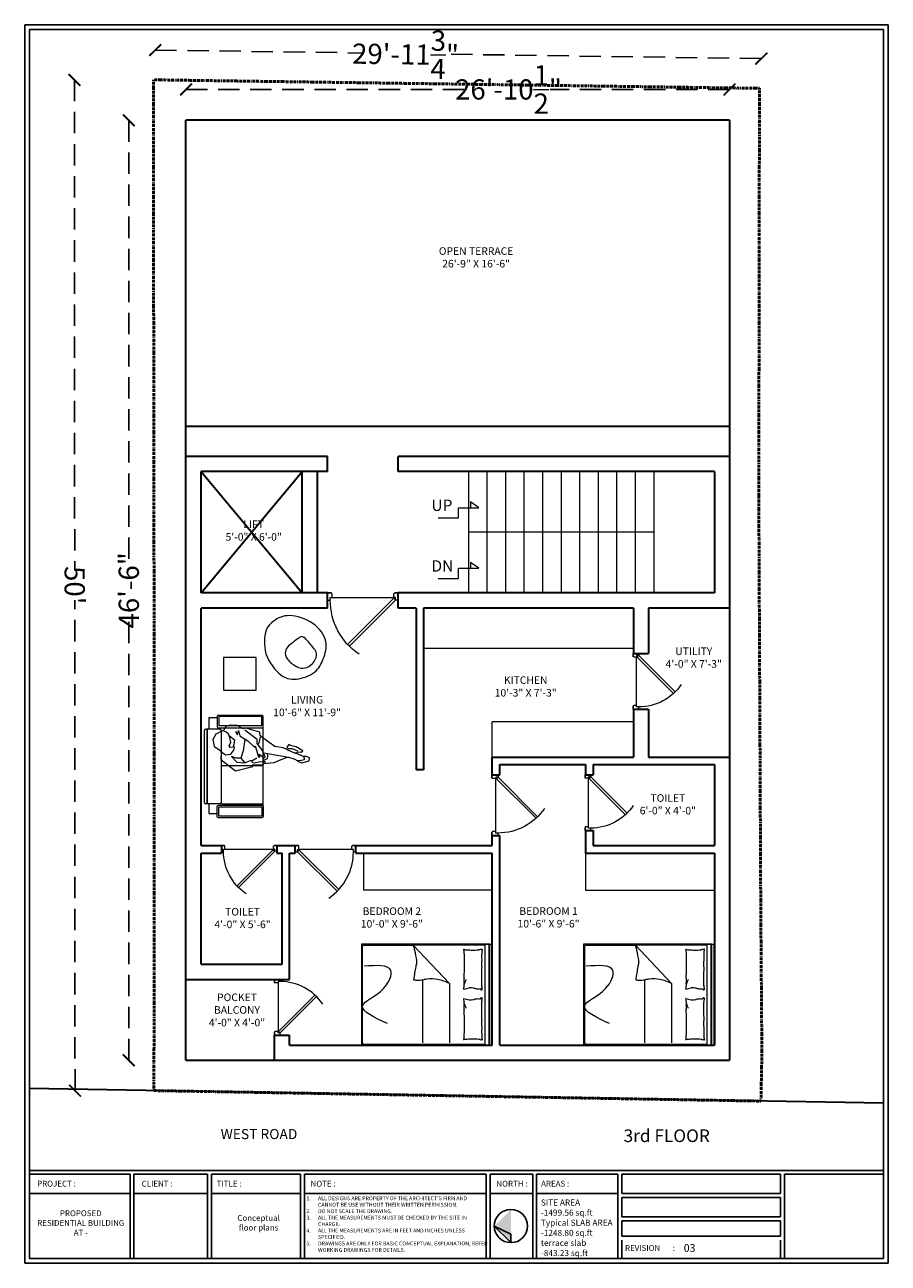
# Model space of a CAD drawing. Units: inches. Extents: x -16911 to -9621, y -48626 to -46270.
# Tile 4 of 20: x -15711 to -15199, y -47065 to -46330. Entities that reach past the tile are written whole.
import ezdxf

# ---------------------------------------------------------------- set-up
doc = ezdxf.new("R2010")
doc.units = ezdxf.units.IN
for name, pattern in [('DASHDOT', [1, 0.5, -0.25, 0, -0.25]), ('DASHED', [19.05, 12.7, -6.35]), ('DOT2', [3.175, 0, -3.175])]:
    doc.linetypes.add(name, pattern=pattern)
for name, color, linetype, lineweight in [('A-ANNO-DIMS', 2, 'Continuous', 13), ('A-ANNO-SYMB', 3, 'Continuous', 13), ('A-ANNO-TEXT', 7, 'Continuous', 18), ('A-ANNO-TTLB', 7, 'Continuous', 25), ('A-AREA-IDEN', 3, 'Continuous', 18), ('A-DOOR', 4, 'Continuous', 18), ('A-FLOR-STRS', 3, 'Continuous', 18), ('A-FURN', 8, 'Continuous', 13), ('A-WALL', 7, 'Continuous', 35), ('C-PROP', 6, 'DASHDOT', 50), ('DOOR', 143, 'Continuous', 9), ('furniture', 35, 'Continuous', 15), ('Man', 8, 'Continuous', 5), ('STAIRCASE', 137, 'Continuous', 5)]:
    doc.layers.add(name, color=color, linetype=linetype, lineweight=lineweight)
doc.styles.get("Standard").update_dxf_attribs({"font": 'swissel.ttf'})
doc.styles.add('style9', font='swisscl.ttf', dxfattribs={"height": 12})
doc.dimstyles.new('Dim9', dxfattribs={"dimtxt": 10, "dimasz": 0.199219, "dimexe": 1, "dimexo": 0.5, "dimgap": 1, "dimtad": 0, "dimdec": 1, "dimzin": 0, "dimdsep": 46, "dimlunit": 4, "dimtxsty": 'style9', "dimblk": 'ARCHTICK', "dimcen": 0.09, "dimclrd": 256, "dimclrt": 256, "dimadec": 0, "dimazin": 0, "dimtfac": 1, "dimtdec": 1, "dimtix": 1, "dimtofl": 0, "dimtmove": 1, "dimatfit": 3, "dimfxl": 9, "dimtolj": 1, "dimtzin": 0, "dimlwd": -1, "dimarcsym": 0})

# ---------------------------------------------------------------- blocks, each defined once
blk = doc.blocks.new('Bipman02')
blk.add_lwpolyline([(0.587, -0.067), (0.618, -0.05), (0.652, -0.054), (0.67, -0.038), (0.596, 0.007), (0.544, 0.016), (0.516, 0.03), (0.496, 0.007), (0.492, -0.023), (0.452, -0.006), (0.357, 0.011), (0.292, 0.055), (0.192, 0.129), (0.187, 0.172), (0.031, 0.216), (0.005, 0.207), (-0.069, 0.246), (-0.147, 0.25), (-0.195, 0.233), (-0.225, 0.181), (-0.238, 0.185), (-0.308, 0.15), (-0.343, 0.09), (-0.325, 0.011), (-0.256, -0.037), (-0.247, -0.058), (-0.251, -0.137), (-0.086, -0.263), (0.109, -0.215), (0.109, -0.193), (0.226, -0.197), (0.231, -0.184), (0.352, -0.171), (0.409, -0.145), (0.487, -0.115), (0.509, -0.11), (0.583, -0.132), (0.609, -0.15), (0.63, -0.164), (0.661, -0.176), (0.744, -0.154), (0.748, -0.119), (0.714, -0.105), (0.674, -0.102), (0.639, -0.084)], close=True)
for points in [[(-0.256, -0.045), (-0.199, -0.084), (-0.138, -0.076), (-0.104, -0.032), (-0.099, 0.007), (-0.147, -0.002), (-0.156, 0.016), (-0.138, 0.059), (-0.151, 0.111), (-0.165, 0.15), (-0.191, 0.172), (-0.217, 0.181)], [(-0.086, 0.177), (-0.065, 0.142), (-0.052, 0.19), (-0.039, 0.129), (0.053, 0.072), (0.127, 0.003), (0.135, 0.016), (0.174, -0.106), (0.187, -0.11), (0.179, -0.076), (0.235, -0.119), (0.248, -0.106), (0.209, -0.023), (0.157, 0.042), (0.157, 0.09), (0.018, 0.194)], [(-0.156, 0.133), (-0.099, 0.085), (-0.104, 0.033), (-0.112, 0.007)], [(0.018, 0.09), (0.001, -0.041), (-0.025, -0.123), (-0.078, -0.123), (-0.13, -0.102), (-0.073, -0.167), (0.014, -0.176), (0.092, -0.145), (0.101, -0.176)], [(0.192, 0.116), (0.174, 0.037)], [(-0.025, -0.123), (0.014, -0.171)], [(0.096, -0.154), (0.153, -0.119)], [(0.27, -0.076), (0.274, -0.097), (0.27, -0.128), (0.244, -0.141), (0.222, -0.145), (0.248, -0.163), (0.248, -0.171), (0.2, -0.163), (0.114, -0.18)], [(0.231, -0.063), (0.361, -0.084), (0.509, -0.109)], [(0.492, -0.023), (0.587, -0.067)], [(0.505, -0.015), (0.552, -0.015), (0.613, -0.041)], [(0.678, -0.11), (0.691, -0.128), (0.687, -0.141), (0.657, -0.15), (0.609, -0.154)]]:
    blk.add_lwpolyline(points)
blk = doc.blocks.new('erertety')
at = {"layer": 'furniture', "ltscale": 0.2}
for p, q in [((-17662.13, -45230.66), (-17662.13, -45176.69)), ((-17693.83, -45223.2), (-17693.83, -45184.43)), ((-17685.49, -45183.68), (-17693.08, -45183.68)), ((-17684.74, -45223.2), (-17684.74, -45184.43)), ((-17684.74, -45203.31), (-17662.13, -45203.31)), ((-17685.49, -45223.95), (-17693.08, -45223.95)), ((-17691.58, -45223.95), (-17691.58, -45229.1)), ((-17684.74, -45223.99), (-17662.13, -45223.99)), ((-17684.74, -45224.55), (-17662.13, -45224.55)), ((-17684.74, -45224.55), (-17662.13, -45224.55)), ((-17691.58, -45229.1), (-17687.09, -45229.1))]:
    blk.add_line(p, q, dxfattribs=at)
blk.add_lwpolyline([(-17687.09, -45177.54), (-17691.58, -45177.54), (-17691.58, -45183.68)], dxfattribs=at)
for points in [[(-17662.13, -45182.17), (-17662.13, -45176.97, 0.414214), (-17662.87, -45176.22), (-17686.34, -45176.22, 0.414214), (-17687.09, -45176.97), (-17687.09, -45182.17, 0.414214), (-17686.34, -45182.91), (-17662.87, -45182.91, 0.414214)], [(-17662.13, -45225.47), (-17662.13, -45230.66, -0.414214), (-17662.87, -45231.41), (-17686.34, -45231.41, -0.414214), (-17687.09, -45230.66), (-17687.09, -45225.47, -0.414214), (-17686.34, -45224.72), (-17662.87, -45224.72, -0.414214)]]:
    blk.add_lwpolyline(points, format="xyb", close=True, dxfattribs=at)
for points in [[(-17663.01, -45181.75), (-17663.01, -45176.82), (-17686.21, -45176.82), (-17686.21, -45181.75)], [(-17692.4, -45183.68), (-17692.4, -45223.95), (-17692.4, -45223.95), (-17692.4, -45183.68)], [(-17663.01, -45225.6), (-17663.01, -45230.53), (-17686.21, -45230.53), (-17686.21, -45225.6)]]:
    blk.add_lwpolyline(points, close=True, dxfattribs=at)
for centre, start, end in [((-17693.08, -45184.43), 90, 180), ((-17685.49, -45184.43), 0, 90), ((-17693.08, -45223.2), 180, 270), ((-17685.49, -45223.2), 270, 0)]:
    blk.add_arc(centre, 0.748, start, end, dxfattribs=at)
at = {"layer": 'furniture', "ltscale": 0.2, "xscale": 47.90818138957024, "yscale": 47.90818138957024, "zscale": 47.90818138957024}
blk.add_blockref('Bipman02', (-17673, -45193.44, 0), dxfattribs=at)
blk = doc.blocks.new('rthrty')
at = {"layer": 'furniture'}
blk.add_open_spline([(-17650.3, -45154.53), (-17651.97, -45142.9), (-17645.3, -45136.31), (-17637.11, -45132.37), (-17620.71, -45137.17), (-17612.47, -45149.45), (-17615.73, -45159.71), (-17619.67, -45168.02), (-17632.28, -45172.65), (-17641.84, -45170.43), (-17649.5, -45159.42), (-17650.3, -45154.53)], degree=3, dxfattribs=at)
at = {"layer": 'Man'}
blk.add_open_spline([(-17632.99, -45149.02), (-17629.89, -45146.6), (-17628, -45145.12), (-17623.29, -45151.15), (-17618.06, -45156.77), (-17623.15, -45164.08), (-17628.28, -45165.32), (-17631.61, -45164.6), (-17638.01, -45159.61), (-17638.81, -45154.69), (-17636.9, -45151.81), (-17632.99, -45149.02), (-17632.99, -45149.02)], degree=3, dxfattribs=at)
blk = doc.blocks.new('hjuyuiuyk')
at = {"layer": 'furniture'}
for p, q in [((-19327.49, -39738.98), (-19327.49, -39737.31)), ((-19327.49, -39737.31), (-19267.49, -39737.31, 0)), ((-19327.49, -39746.54), (-19327.49, -39737.31)), ((-19267.49, -39738.5), (-19327.49, -39738.5, 0)), ((-19327.49, -39738.5, 0), (-19327.49, -39814.72, 0)), ((-19327.49, -39738.5), (-19327.49, -39814.72)), ((-19267.49, -39738.5, 0), (-19327.49, -39738.5)), ((-19267.49, -39738.98, 0), (-19327.49, -39738.98)), ((-19268.1, -39741.33), (-19326.9, -39741.33)), ((-19326.9, -39741.33), (-19326.9, -39813.21)), ((-19268.1, -39813.21), (-19268.1, -39741.33)), ((-19267.49, -39737.31, 0), (-19267.49, -39738.98, 0)), ((-19267.49, -39746.54, 0), (-19267.49, -39737.31, 0)), ((-19267.49, -39814.72), (-19267.49, -39738.5)), ((-19267.49, -39814.72, 0), (-19267.49, -39738.5, 0)), ((-19300.88, -39753.22, 0), (-19301.49, -39750.81, 0)), ((-19300.67, -39754.09, 0), (-19300.88, -39753.22, 0)), ((-19295.19, -39754.09, 0), (-19294.97, -39753.22, 0)), ((-19294.97, -39753.22, 0), (-19294.37, -39750.81, 0)), ((-19304.07, -39762.52), (-19326.9, -39783.91)), ((-19304.07, -39762.52), (-19268.82, -39762.52)), ((-19268.82, -39778.34), (-19306.29, -39778.34)), ((-19326.9, -39813.21), (-19326.9, -39783.91)), ((-19327.49, -39814.72, 0), (-19267.49, -39814.72)), ((-19327.49, -39814.72), (-19267.49, -39814.72, 0)), ((-19269.1, -39814.21), (-19325.9, -39814.21)), ((-19325.9, -39814.21), (-19269.1, -39814.21))]:
    blk.add_line(p, q, dxfattribs=at)
for centre, radius, start, end in [((-19324.36, -39743.07, 0), 0.0997, 111.7883, 160.43603), ((-19324.39, -39743.06, 0), 0.0676, 160.43603, 281.89306), ((-19324.12, -39743.66, 0), 0.732, 94.30254, 111.7883), ((-19324.35, -39743.25, 0), 0.125, 21.9904, 101.89306), ((-19323.34, -39743.89, 0), 0.956, 158.57902, 188.13348), ((-19317.18, -39743.01, 0), 7.17, 188.13348, 192.10946), ((-19324.65, -39743.37, 0), 0.455, 338.57902, 21.9904), ((-19329.85, -39745.73, 0), 5.78, 7.6809, 12.10946), ((-19324.11, -39743.77, 0), 0.842, 59.34875, 94.30254), ((-19350.51, -39748.51, 0), 26.62, 3.36875, 7.6809), ((-19363.7, -39747.54, 0), 39.81, 356.94504, 358.36691), ((-19343.69, -39748.11, 0), 19.79, 358.36691, 3.36875), ((-19322.88, -39741.69, 0), 1.57, 239.34875, 264.74081), ((-19319.6, -39692.5, 0), 50.87, 266.13994, 268.60024), ((-19319.84, -39713.09, 0), 30.28, 268.09211, 271.28082), ((-19320.24, -39695.07, 0), 48.31, 271.28082, 273.40341), ((-19316.15, -39763.89, 0), 20.63, 90.1553, 93.40341), ((-19316.09, -39783.15, 0), 39.89, 86.99024, 90.1553), ((-19305.86, -39588.51, 0), 155.02, 266.99024, 268.59569), ((-19305.42, -39570.46, 0), 173.07, 268.59569, 270), ((-19305.42, -39718.38, 0), 25.15, 270, 273.68415), ((-19304.03, -39739.9, 0), 3.58, 273.68415, 287.19507), ((-19300.46, -39751.46, 0), 8.51, 98.43719, 107.19507), ((-19301.02, -39747.69, 0), 4.7, 90, 98.43719), ((-19282.35, -39751.13, 0), 19.21, 171.99495, 177.33512), ((-19292.22, -39749.75, 0), 9.25, 167.80162, 171.99495), ((-19326.4, -39742.36, 0), 25.72, 347.80162, 350.31563), ((-19301.12, -39743.14, 0), 0.997, 274.40021, 333.41948), ((-19315.3, -39745.68, 0), 14.34, 360, 6.23236), ((-19306.91, -39745.68, 0), 5.95, 350.31563, 360), ((-19301.02, -39745.63, 0), 2.64, 78.72762, 90), ((-19300.58, -39743.42, 0), 0.383, 333.41948, 78.72762), ((-19295.28, -39743.42, 0), 0.383, 101.27238, 206.58052), ((-19294.73, -39743.14, 0), 0.997, 206.58052, 265.59979), ((-19294.84, -39745.63, 0), 2.64, 90, 101.27238), ((-19280.55, -39745.68, 0), 14.34, 173.76764, 180), ((-19288.94, -39745.68, 0), 5.95, 180, 189.68437), ((-19294.84, -39747.69, 0), 4.7, 81.56281, 90), ((-19269.45, -39742.36, 0), 25.72, 189.68437, 192.19838), ((-19303.63, -39749.75, 0), 9.25, 8.00505, 12.19838), ((-19313.5, -39751.13, 0), 19.21, 2.66488, 8.00505), ((-19295.39, -39751.46, 0), 8.51, 72.80493, 81.56281), ((-19291.82, -39739.9, 0), 3.58, 252.80493, 266.31585), ((-19290.43, -39718.38, 0), 25.15, 266.31585, 270), ((-19290.43, -39570.46, 0), 173.07, 270, 271.40431), ((-19289.99, -39588.51, 0), 155.02, 271.40431, 273.00976), ((-19279.76, -39783.15, 0), 39.89, 89.8447, 93.00976), ((-19279.7, -39763.89, 0), 20.63, 86.59659, 89.8447), ((-19275.61, -39695.07, 0), 48.31, 266.59659, 268.71918), ((-19276.02, -39713.09, 0), 30.28, 268.71918, 271.90789), ((-19276.73, -39645.13, 0), 98.25, 271.00686, 272.7772), ((-19272.12, -39741.69, 0), 1.57, 275.25919, 300.65125), ((-19270.89, -39743.77, 0), 0.842, 85.69746, 120.65125), ((-19251.31, -39748.11, 0), 19.79, 176.63125, 181.63309), ((-19231.3, -39747.54, 0), 39.81, 181.63309, 183.05496), ((-19244.49, -39748.51, 0), 26.62, 172.3191, 176.63125), ((-19265.15, -39745.73, 0), 5.78, 167.89054, 172.3191), ((-19270.88, -39743.66, 0), 0.732, 68.2117, 85.69746), ((-19270.35, -39743.37, 0), 0.455, 158.0096, 201.42098), ((-19277.82, -39743.01, 0), 7.17, 347.89054, 351.86652), ((-19270.65, -39743.25, 0), 0.125, 78.10694, 158.0096), ((-19271.66, -39743.89, 0), 0.956, 351.86652, 21.42098), ((-19270.61, -39743.06, 0), 0.0676, 258.10694, 19.56397), ((-19270.64, -39743.07, 0), 0.0997, 19.56397, 68.2117), ((-19323.69, -39753.93, 0), 0.564, 170.00164, 196.69777), ((-19333.47, -39752.21, 0), 9.37, 350.00164, 356.49514), ((-19324.19, -39754.08, 0), 0.0385, 196.69777, 277.12039), ((-19324.51, -39751.59, 0), 2.55, 277.12039, 286.22115), ((-19720.99, -39728.47, 0), 397.61, 356.49514, 356.94504), ((-19324.42, -39751.9, 0), 2.23, 286.22115, 297.44392), ((-19322.81, -39754.99, 0), 1.25, 102.44799, 117.44392), ((-19322.32, -39757.22, 0), 3.54, 93.57397, 102.44799), ((-19318.44, -39837.61, 0), 84.03, 90.97549, 92.79548), ((-19315.55, -39952.16, 0), 198.61, 89.44614, 91.24735), ((-19314.9, -39885.06, 0), 131.51, 87.23256, 89.44614), ((-19310.57, -39795.48, 0), 41.81, 85.40123, 87.23256), ((-19304.32, -39717.78, 0), 36.14, 265.40123, 267.37117), ((-19297.32, -39733.09, 0), 21.54, 244.68893, 246.51559), ((-19305.66, -39747.05, 0), 6.83, 267.37117, 281.48268), ((-19297.32, -39733.09, 0), 21.54, 246.51559, 248.34226), ((-19297.32, -39733.09, 0), 21.54, 248.34226, 250.57202), ((-19297.32, -39733.09, 0), 21.54, 250.57202, 252.80178), ((-19303.46, -39757.91, 0), 4.25, 83.56595, 101.48268), ((-19303.37, -39757.16, 0), 3.49, 72.61359, 83.56595), ((-19300.33, -39747.43, 0), 6.7, 252.61359, 260.5159), ((-19299.57, -39750.33, 0), 1.97, 177.33512, 194.04519), ((-19300.13, -39746.25, 0), 7.9, 260.5159, 265.91706), ((-19300.69, -39754.1, 0), 0.0267, 265.91706, 14.04494), ((-19295.16, -39754.1, 0), 0.0267, 165.95506, 274.08294), ((-19295.72, -39746.25, 0), 7.9, 274.08294, 279.4841), ((-19295.52, -39747.43, 0), 6.7, 279.4841, 287.38641), ((-19296.28, -39750.33, 0), 1.97, 345.95481, 2.66488), ((-19292.48, -39757.16, 0), 3.49, 96.43405, 107.38641), ((-19292.39, -39757.91, 0), 4.25, 78.51732, 96.43405), ((-19298.54, -39733.09, 0), 21.54, 287.19822, 289.42798), ((-19290.19, -39747.05, 0), 6.83, 258.51732, 272.62883), ((-19298.54, -39733.09, 0), 21.54, 289.42798, 291.65774), ((-19298.54, -39733.09, 0), 21.54, 291.65774, 293.48441), ((-19298.54, -39733.09, 0), 21.54, 293.48441, 295.31107), ((-19291.53, -39717.78, 0), 36.14, 272.62883, 274.59877), ((-19285.28, -39795.48, 0), 41.81, 92.76744, 94.59877), ((-19280.95, -39885.06, 0), 131.51, 90.55386, 92.76744), ((-19280.3, -39952.16, 0), 198.61, 88.75265, 90.55386), ((-19277.1, -39805.01, 0), 51.42, 86.42603, 88.75265), ((-19274.68, -39799.75, 0), 46.07, 86.55746, 89.01709), ((-19272.19, -39754.99, 0), 1.25, 62.55608, 77.55201), ((-19270.58, -39751.9, 0), 2.23, 242.55608, 253.77885), ((-19270.49, -39751.59, 0), 2.55, 253.77885, 262.87961), ((-18874.01, -39728.47, 0), 397.61, 183.05496, 183.50486), ((-19261.53, -39752.21, 0), 9.37, 183.50486, 189.99836), ((-19270.81, -39754.08, 0), 0.0385, 262.87961, 343.30223), ((-19271.31, -39753.93, 0), 0.564, 343.30223, 9.99836), ((-19279.47, -39774.89), 27.53, 153.30845, 168.74227), ((-19287.94, -39773.2), 18.89, 168.74227, 187.39945), ((-19242.78, -39767.34), 64.43, 187.39945, 189.27191), ((-19333.07, -39782.08), 27.05, 6.38169, 9.27191), ((-19306.77, -39846.83), 66.07, 105.93519, 107.73639), ((-19318.41, -39806.06), 23.67, 102.92554, 105.93519), ((-19287.64, -39956.87), 177.57, 99.72434, 101.71957), ((-19317.24, -39783.9), 2.09, 82.26962, 100.72756), ((-19317.9, -39788.76), 6.99, 76.8096, 82.26962), ((-19295.64, -39693.77), 90.57, 256.8096, 258.32586), ((-19295.11, -39691.23), 93.17, 258.32586, 260.50498), ((-19288.03, -39648.9), 136.08, 260.50498, 262.308), ((-19336.71, -39780.62), 30.63, 354.11415, 359.23133), ((-19321.79, -39780.82), 15.7, 359.23133, 6.38169), ((-19325.9, -39813.21), 1, 180, 270), ((-19269.1, -39813.21), 1, 270, 0)]:
    blk.add_arc(centre, radius, start, end, dxfattribs=at)
blk.add_open_spline([(-19280.24, -39799.21), (-19283.87, -39806.94), (-19290.73, -39821.55), (-19298.08, -39801.09), (-19315.85, -39793.47), (-19314.86, -39805.92), (-19314.29, -39813.13)], degree=3, knots=[0, 0, 0, 0, 18.167809, 34.338432, 45.972904, 61.997799, 61.997799, 61.997799, 61.997799], dxfattribs=at)
blk = doc.blocks.new('A$C1C9D3E54')
at = {"layer": 'DOOR'}
blk.add_line((18676.53, 5780.72), (18710.53, 5780.72), dxfattribs=at)
blk.add_lwpolyline([(18685.01, 5806.62), (18710.47, 5781.16), (18711.53, 5782.22), (18686.07, 5807.68), (18685.01, 5806.62)], dxfattribs=at)
blk.add_lwpolyline([(18674.03, 5778.22), (18676.03, 5778.22), (18674.03, 5778.22), (18674.03, 5782.22), (18675.53, 5782.22), (18675.53, 5780.72), (18676.53, 5780.72), (18676.53, 5778.72), (18676.41, 5778.72), (18676.41, 5778.6, -0.414214), (18676.16, 5778.35), (18676.03, 5778.35), (18676.03, 5778.22)], format="xyb", dxfattribs=at)
blk.add_lwpolyline([(18713.03, 5782.22), (18711.53, 5782.22), (18711.53, 5780.72), (18710.53, 5780.72), (18710.53, 5778.72), (18710.66, 5778.72), (18710.66, 5778.6, 0.414214), (18710.91, 5778.35), (18711.03, 5778.35), (18711.03, 5778.22), (18713.03, 5778.22), (18711.03, 5778.22), (18713.03, 5778.22), (18713.03, 5782.22)], format="xyb", close=True, dxfattribs=at)
blk.add_arc((18711.53, 5782.22), 36, 124.03362, 180, dxfattribs=at)
blk = doc.blocks.new('_ArchTick')
at = {"color": 0, "linetype": 'ByBlock', "const_width": 0.15}
blk.add_lwpolyline([(-0.5, -0.5), (0.5, 0.5)], dxfattribs=at)
blk = doc.blocks.new('*D61')
at = {"layer": 'A-ANNO-DIMS', "color": 0, "linetype": 'DOT2', "lineweight": -2, "transparency": 16777216}
for p, q in [((-15634.02, -46345.34), (-15634, -46344.15)), ((-15274.35, -46350.39), (-15274.34, -46349.2))]:
    blk.add_line(p, q, dxfattribs=at)
at = {"layer": 'A-ANNO-DIMS', "color": 0, "linetype": 'DASHED', "lineweight": 25, "transparency": 16777216}
for p, q in [((-15634.01, -46345.15), (-15510.27, -46346.89)), ((-15274.35, -46350.2), (-15460.69, -46347.59))]:
    blk.add_line(p, q, dxfattribs=at)
at = {"layer": 'Defpoints', "color": 0, "transparency": 16777216}
for p in [(-15274.35, -46350.2), (-15634.21, -46359.07), (-15274.55, -46364.11)]:
    blk.add_point(p, dxfattribs=at)
at = {"layer": 'A-ANNO-DIMS', "color": 0, "lineweight": 25, "transparency": 16777216, "xscale": 7, "yscale": 7, "zscale": 7}
for p, rotation in [((-15634.01, -46345.15), 179.1963905603631), ((-15274.35, -46350.2), 359.196390560363)]:
    blk.add_blockref('_ArchTick', p, dxfattribs=dict(at, rotation=rotation))
at = {"layer": 'A-ANNO-DIMS', "color": 0, "transparency": 16777216, "insert": (-15485.49, -46347.68), "char_height": 12, "attachment_point": 5, "rotation": 359.19639, "style": 'style9'}
blk.add_mtext('\\A1;29\'-11{\\H1x;\\S3/4;}"', dxfattribs=at)
blk = doc.blocks.new('*D62')
at = {"layer": 'A-ANNO-DIMS', "color": 0, "linetype": 'DOT2', "lineweight": -2, "transparency": 16777216}
for p, q in [((-15681.81, -46362.82), (-15683, -46362.82)), ((-15681.44, -46962.82), (-15682.63, -46962.82))]:
    blk.add_line(p, q, dxfattribs=at)
at = {"layer": 'A-ANNO-DIMS', "color": 0, "linetype": 'DASHED', "lineweight": 25, "transparency": 16777216}
for p, q in [((-15682, -46362.82), (-15681.82, -46653.98)), ((-15681.63, -46962.82), (-15681.81, -46671.67))]:
    blk.add_line(p, q, dxfattribs=at)
at = {"layer": 'Defpoints', "color": 0, "transparency": 16777216}
for p in [(-15682, -46362.82), (-15663.18, -46362.81), (-15662.82, -46962.81)]:
    blk.add_point(p, dxfattribs=at)
at = {"layer": 'A-ANNO-DIMS', "color": 0, "lineweight": 25, "transparency": 16777216, "xscale": 7, "yscale": 7, "zscale": 7}
for p, rotation in [((-15682, -46362.82), 90.0346840750536), ((-15681.63, -46962.82), 270.0346840750536)]:
    blk.add_blockref('_ArchTick', p, dxfattribs=dict(at, rotation=rotation))
at = {"layer": 'A-ANNO-DIMS', "color": 0, "transparency": 16777216, "insert": (-15681.81, -46662.82), "char_height": 12, "attachment_point": 5, "rotation": 270.03468, "style": 'style9'}
blk.add_mtext("\\A1;50'", dxfattribs=at)
blk = doc.blocks.new('*D63')
at = {"layer": 'A-ANNO-DIMS', "color": 0, "linetype": 'DOT2', "lineweight": -2, "transparency": 16777216}
for p, q in [((-15615.78, -46368.33), (-15615.78, -46369.52)), ((-15293.23, -46368.33), (-15293.23, -46369.52))]:
    blk.add_line(p, q, dxfattribs=at)
at = {"layer": 'A-ANNO-DIMS', "color": 0, "linetype": 'DASHED', "lineweight": 25, "transparency": 16777216}
for p, q in [((-15615.78, -46368.52), (-15449, -46368.52)), ((-15293.23, -46368.52), (-15399.73, -46368.52))]:
    blk.add_line(p, q, dxfattribs=at)
at = {"layer": 'Defpoints', "color": 0, "transparency": 16777216}
for p in [(-15615.78, -46345.28), (-15293.23, -46345.28), (-15293.23, -46368.52)]:
    blk.add_point(p, dxfattribs=at)
at = {"layer": 'A-ANNO-DIMS', "color": 0, "lineweight": 25, "transparency": 16777216, "xscale": 7, "yscale": 7, "zscale": 7, "rotation": 180}
blk.add_blockref('_ArchTick', (-15615.78, -46368.52), dxfattribs=at)
at = {"layer": 'A-ANNO-DIMS', "color": 0, "lineweight": 25, "transparency": 16777216, "xscale": 7, "yscale": 7, "zscale": 7}
blk.add_blockref('_ArchTick', (-15293.23, -46368.52), dxfattribs=at)
at = {"layer": 'A-ANNO-DIMS', "color": 0, "transparency": 16777216, "insert": (-15424.37, -46368.52), "char_height": 12, "attachment_point": 5, "style": 'style9'}
blk.add_mtext('\\A1;26\'-10{\\H1x;\\S1/2;}"', dxfattribs=at)
blk = doc.blocks.new('*D64')
at = {"layer": 'A-ANNO-DIMS', "color": 0, "linetype": 'DOT2', "lineweight": -2, "transparency": 16777216}
for p, q in [((-15649.52, -46386.86), (-15650.71, -46386.86)), ((-15649.52, -46944.81), (-15650.71, -46944.81))]:
    blk.add_line(p, q, dxfattribs=at)
at = {"layer": 'A-ANNO-DIMS', "color": 0, "linetype": 'DASHED', "lineweight": 25, "transparency": 16777216}
for p, q in [((-15649.71, -46386.86), (-15649.71, -46648.2)), ((-15649.71, -46944.81), (-15649.71, -46683.47))]:
    blk.add_line(p, q, dxfattribs=at)
at = {"layer": 'Defpoints', "color": 0, "transparency": 16777216}
for p in [(-15615.78, -46386.86), (-15649.71, -46944.81), (-15615.78, -46944.81)]:
    blk.add_point(p, dxfattribs=at)
at = {"layer": 'A-ANNO-DIMS', "color": 0, "lineweight": 25, "transparency": 16777216, "xscale": 7, "yscale": 7, "zscale": 7}
for p, rotation in [((-15649.71, -46386.86), 90), ((-15649.71, -46944.81), 270)]:
    blk.add_blockref('_ArchTick', p, dxfattribs=dict(at, rotation=rotation))
at = {"layer": 'A-ANNO-DIMS', "color": 0, "transparency": 16777216, "insert": (-15649.71, -46665.83), "char_height": 12, "attachment_point": 5, "rotation": 90, "style": 'style9'}
blk.add_mtext('\\A1;46\'-6"', dxfattribs=at)
blk = doc.blocks.new('THYHYTJ')
at = {"layer": 'STAIRCASE', "ltscale": 10}
for p, q in [((-7981.18, -46346.18), (-7984.62, -46351.1)), ((-7981.18, -46358.18), (-7981.18, -46346.18)), ((-7984.62, -46351.1), (-7981.18, -46351.1)), ((-7975.18, -46358.18), (-7981.18, -46358.18)), ((-7975.18, -46370.18), (-7975.18, -46358.18))]:
    blk.add_line(p, q, dxfattribs=at)
blk = doc.blocks.new('TITLE-BLOCK-A3')
blk.add_hatch(color=256).paths.add_polyline_path([(-16032.81, -47043.2), (-16022.97, -47033.35), (-16022.97, -47053.05)])
for p, q in [((-16311.44, -47065.27), (-16311.44, -46330.13)), ((-16311.44, -46330.13), (-15799.07, -46330.13)), ((-16308.66, -47062.49), (-16308.66, -46332.91)), ((-16308.66, -46332.91), (-15801.86, -46332.91)), ((-15801.86, -46332.91), (-15801.86, -47062.49)), ((-15799.07, -46330.13), (-15799.07, -47065.27)), ((-15801.86, -47010.14), (-16308.66, -47010.14)), ((-16248.93, -47012.43), (-16308.66, -47012.43)), ((-16248.93, -47062.49), (-16248.93, -47012.43)), ((-16202.98, -47012.43), (-16246.63, -47012.43)), ((-16246.63, -47062.49), (-16246.63, -47012.43)), ((-16202.98, -47062.49), (-16202.98, -47012.43)), ((-16147.85, -47012.43), (-16200.68, -47012.43)), ((-16200.68, -47062.49), (-16200.68, -47012.43)), ((-16147.85, -47062.49), (-16147.85, -47012.43)), ((-16037.57, -47012.43), (-16145.55, -47012.43)), ((-16145.55, -47062.49), (-16145.55, -47012.43)), ((-16037.57, -47062.49), (-16037.57, -47012.43)), ((-16010.01, -47012.43), (-16035.28, -47012.43)), ((-16035.28, -47062.49), (-16035.28, -47012.43)), ((-16010.01, -47062.49), (-16010.01, -47012.43)), ((-15959.47, -47012.43), (-16007.71, -47012.43)), ((-16007.71, -47062.49), (-16007.71, -47012.43)), ((-15959.47, -47062.49), (-15959.47, -47012.43)), ((-15862.98, -47012.43), (-15957.17, -47012.43)), ((-15957.17, -47023.95), (-15957.17, -47012.43)), ((-15862.98, -47023.95), (-15862.98, -47012.43)), ((-15801.86, -47012.43), (-15860.68, -47012.43)), ((-15860.68, -47062.49), (-15860.68, -47012.43)), ((-16308.66, -47023.95), (-16248.93, -47023.95)), ((-16246.63, -47023.95), (-16202.98, -47023.95)), ((-16200.68, -47023.95), (-16147.85, -47023.95)), ((-16145.55, -47023.95), (-16037.57, -47023.95)), ((-16035.28, -47023.95), (-16010.01, -47023.95)), ((-16007.71, -47023.95), (-15959.47, -47023.95)), ((-15957.17, -47023.95), (-15862.98, -47023.95)), ((-15957.17, -47037.77), (-15957.17, -47026.25)), ((-15957.17, -47026.25), (-15862.98, -47026.25)), ((-15862.98, -47037.77), (-15862.98, -47026.25)), ((-15957.17, -47037.77), (-15862.98, -47037.77)), ((-15957.17, -47049.29), (-15957.17, -47040.07)), ((-15957.17, -47040.07), (-15862.98, -47040.07)), ((-15862.98, -47049.29), (-15862.98, -47040.07)), ((-15957.17, -47049.29), (-15862.98, -47049.29)), ((-15957.17, -47062.49), (-15957.17, -47051.59)), ((-15862.98, -47062.49), (-15862.98, -47051.59)), ((-15801.86, -47062.49), (-16308.66, -47062.49)), ((-15799.07, -47065.27), (-16311.44, -47065.27))]:
    blk.add_line(p, q)
blk.add_lwpolyline([(-16032.81, -47043.2), (-16022.97, -47047.92), (-16022.97, -47053.05), (-16032.81, -47043.2)])
blk.add_circle((-16022.97, -47043.2), 9.85)

msp = doc.modelspace()

# ---------------------------------------------------------------- linework, layer by layer
at = {"layer": 'A-FLOR-STRS', "ltscale": 10}
for p, q in [((-15448.233, -46595.355), (-15448.233, -46667.355)), ((-15437.233, -46595.355), (-15437.233, -46667.355)), ((-15426.233, -46595.355), (-15426.233, -46667.355)), ((-15415.233, -46595.355), (-15415.233, -46667.355)), ((-15404.233, -46595.355), (-15404.233, -46667.355)), ((-15393.233, -46595.355), (-15393.233, -46667.355)), ((-15382.233, -46595.355), (-15382.233, -46667.355)), ((-15371.233, -46595.355), (-15371.233, -46667.355)), ((-15360.233, -46595.355), (-15360.233, -46667.355)), ((-15349.233, -46595.355), (-15349.233, -46667.355)), ((-15338.233, -46595.355), (-15338.233, -46667.355)), ((-15338.233, -46631.355), (-15448.233, -46631.355))]:
    msp.add_line(p, q, dxfattribs=at)
at = {"layer": 'A-FURN', "ltscale": 0.2}
for p, q in [((-15350.233, -46700.355), (-15474.783, -46700.355)), ((-15350.233, -46743.809), (-15434.033, -46743.809)), ((-15434.033, -46764.809), (-15434.033, -46743.809)), ((-15510.533, -46821.809, 0), (-15510.533, -46843.809, 0)), ((-15378.733, -46821.809), (-15378.733, -46843.809)), ((-15434.033, -46843.809), (-15510.533, -46843.809)), ((-15378.733, -46843.809), (-15302.233, -46843.809))]:
    msp.add_line(p, q, dxfattribs=at)
at = {"layer": 'A-FURN'}
msp.add_lwpolyline([(-15574.187, -46705.751), (-15593.547, -46705.751), (-15593.547, -46725.111), (-15574.187, -46725.111)], close=True, dxfattribs=at)
at = {"layer": 'A-WALL'}
for p, q in [((-15293.233, -46386.855), (-15615.783, -46386.855)), ((-15615.783, -46586.355), (-15615.783, -46386.855)), ((-15293.233, -46386.855), (-15293.233, -46586.355)), ((-15615.783, -46568.355), (-15293.233, -46568.355)), ((-15615.783, -46896.809), (-15615.783, -46586.355)), ((-15531.783, -46586.355), (-15615.783, -46586.355)), ((-15531.783, -46595.355), (-15531.783, -46586.355)), ((-15293.233, -46586.355), (-15489.783, -46586.355)), ((-15489.783, -46595.355), (-15489.783, -46586.355)), ((-15293.233, -46586.355), (-15293.233, -46676.355)), ((-15606.783, -46667.355), (-15606.783, -46595.355)), ((-15531.783, -46595.355), (-15606.783, -46595.355)), ((-15606.783, -46595.355), (-15546.783, -46667.355)), ((-15606.783, -46667.355), (-15546.783, -46595.355)), ((-15546.783, -46667.355), (-15546.783, -46595.355)), ((-15537.783, -46667.355), (-15537.783, -46595.355)), ((-15302.233, -46595.355), (-15489.783, -46595.355)), ((-15302.233, -46595.355), (-15302.233, -46667.355)), ((-15531.783, -46667.355), (-15606.783, -46667.355)), ((-15531.783, -46676.355), (-15531.783, -46667.355)), ((-15302.233, -46667.355), (-15489.783, -46667.355)), ((-15489.783, -46676.355), (-15489.783, -46667.355)), ((-15606.783, -46817.309), (-15606.783, -46676.355)), ((-15531.783, -46676.355), (-15606.783, -46676.355)), ((-15479.283, -46676.355), (-15489.783, -46676.355)), ((-15479.283, -46676.355), (-15479.283, -46772.355)), ((-15350.233, -46676.355), (-15474.783, -46676.355)), ((-15474.783, -46676.355), (-15474.783, -46772.355)), ((-15350.233, -46676.355), (-15350.233, -46703.355)), ((-15293.233, -46676.355), (-15341.233, -46676.355)), ((-15341.233, -46676.355), (-15341.233, -46703.355)), ((-15293.233, -46676.355), (-15293.233, -46764.809)), ((-15350.233, -46703.355), (-15341.233, -46703.355)), ((-15350.233, -46736.355), (-15350.233, -46764.809)), ((-15350.233, -46736.355), (-15341.233, -46736.355)), ((-15341.233, -46736.355), (-15341.233, -46764.809)), ((-15434.033, -46775.309), (-15434.033, -46764.809)), ((-15434.033, -46764.809), (-15350.233, -46764.809)), ((-15429.533, -46775.309), (-15429.533, -46769.309)), ((-15429.533, -46769.309), (-15378.733, -46769.309)), ((-15378.733, -46769.309), (-15378.733, -46775.309)), ((-15374.233, -46769.309), (-15374.233, -46775.309)), ((-15374.233, -46769.309), (-15302.233, -46769.309)), ((-15341.233, -46764.809), (-15293.233, -46764.809)), ((-15302.233, -46769.309), (-15302.233, -46817.309)), ((-15293.233, -46764.809), (-15293.233, -46944.809)), ((-15474.783, -46772.355), (-15479.283, -46772.355)), ((-15434.033, -46775.309), (-15429.533, -46775.309)), ((-15378.733, -46775.309), (-15374.233, -46775.309)), ((-15434.033, -46817.309), (-15434.033, -46811.309)), ((-15434.033, -46811.309), (-15429.533, -46811.309)), ((-15429.533, -46935.809), (-15429.533, -46811.309)), ((-15378.733, -46808.309), (-15378.733, -46821.809)), ((-15378.733, -46808.309), (-15374.233, -46808.309)), ((-15374.233, -46808.309), (-15374.233, -46817.309)), ((-15606.783, -46817.309), (-15594.783, -46817.309)), ((-15594.783, -46817.309), (-15594.783, -46821.809)), ((-15561.783, -46817.309), (-15551.033, -46817.309)), ((-15561.783, -46817.309), (-15561.783, -46821.809)), ((-15551.033, -46821.809), (-15551.033, -46817.309)), ((-15515.033, -46817.309), (-15434.033, -46817.309)), ((-15515.033, -46821.809), (-15515.033, -46817.309)), ((-15374.233, -46817.309), (-15302.233, -46817.309)), ((-15606.783, -46887.809), (-15606.783, -46821.809)), ((-15606.783, -46821.809), (-15594.783, -46821.809)), ((-15561.783, -46821.809), (-15558.783, -46821.809)), ((-15558.783, -46887.809), (-15558.783, -46821.809)), ((-15554.283, -46896.809), (-15554.283, -46821.809)), ((-15554.283, -46821.809), (-15551.033, -46821.809)), ((-15515.033, -46821.809), (-15434.033, -46821.809)), ((-15434.033, -46935.809), (-15434.033, -46821.809)), ((-15378.733, -46821.809), (-15302.233, -46821.809)), ((-15302.233, -46821.809), (-15302.233, -46935.809)), ((-15606.783, -46887.809), (-15558.783, -46887.809)), ((-15615.783, -46944.809), (-15615.783, -46896.809)), ((-15615.783, -46896.809), (-15554.283, -46896.809)), ((-15563.283, -46944.809), (-15563.283, -46929.809)), ((-15563.283, -46929.809), (-15554.283, -46929.809)), ((-15554.283, -46935.809), (-15554.283, -46929.809)), ((-15554.283, -46935.809), (-15434.033, -46935.809)), ((-15429.533, -46935.809), (-15302.233, -46935.809)), ((-15615.783, -46944.809), (-15563.283, -46944.809)), ((-15563.283, -46944.809), (-15293.233, -46944.809)), ((-15201.856, -46970.292), (-15708.658, -46961.533))]:
    msp.add_line(p, q, dxfattribs=at)
at = {"layer": 'C-PROP'}
msp.add_lwpolyline([(-15634.783, -46962.809), (-15274.601, -46969.035), (-15274.04, -46940.446), (-15274.703, -46855.606), (-15275.869, -46609.511), (-15275.483, -46367.855), (-15635.146, -46362.811), (-15634.608, -46762.955)], close=True, dxfattribs=at)

# ---------------------------------------------------------------- block references
at = {"layer": 'A-ANNO-SYMB', "rotation": 270.0000000000144}
for p in [(30904.121, -54597.957), (30904.121, -54633.957)]:
    msp.add_blockref('THYHYTJ', p, dxfattribs=at)
at = {"layer": 'A-ANNO-TTLB'}
msp.add_blockref('TITLE-BLOCK-A3', (600, 0), dxfattribs=at)
at = {"layer": 'A-DOOR'}
for p, xscale, yscale, zscale, rotation in [((-35642.277, -40444.653), -1.076923076922859, 1.076923076922859, 1.076923076922859, 180), ((-20239.75, -62537.458), -0.8461538461538624, 0.8461538461538624, 0.8461538461538624, 270), ((-20768.028, -64048.876), -0.9230769230769229, 0.9230769230769229, 0.9230769230769229, 270), ((-20268.25, -62609.412), -0.8461538461538624, 0.8461538461538624, 0.8461538461538624, 270), ((-31395.886, -41928.043), -0.8461538461538624, 0.8461538461538624, 0.8461538461538624, 180), ((1722.534, -41483.564), 0.9230769230769229, 0.9230769230769229, 0.9230769230769229, 180), ((-20452.549, -31095.706), 0.8461538461538624, 0.8461538461538624, 0.8461538461538624, 270)]:
    msp.add_blockref('A$C1C9D3E54', p, dxfattribs=dict(at, xscale=xscale, yscale=yscale, zscale=zscale, rotation=rotation))
at = {"layer": 'A-FURN'}
msp.add_blockref('rthrty', (2081.543, -1547.053), dxfattribs=at)
at = {"layer": 'A-FURN', "xscale": 1.1, "yscale": 1.1, "zscale": 1.1}
msp.add_blockref('erertety', (3858.451, 2953.75, 0), dxfattribs=at)
at = {"layer": 'A-FURN', "rotation": 270}
for p in [(24303.029, -66203.296), (24434.829, -66203.296, 0)]:
    msp.add_blockref('hjuyuiuyk', p, dxfattribs=at)

# ---------------------------------------------------------------- texts
at = {"layer": 'A-ANNO-TEXT'}
for s, p in [('UP', (-15470.133, -46618.742)), ('DN', (-15470.133, -46654.742))]:
    msp.add_text(s, height=6.75, dxfattribs=at).set_placement(p)
at = {"layer": 'A-ANNO-TEXT', "ltscale": 10, "style": 'style9'}
for s, insert, char_height, width, attachment_point in [('\\A1;{\\fCentury Gothic|b0|i0|c0|p34;WEST ROAD}', (-15595.193, -46985.611), 6, 70.69764, 1), ('\\A1;{\\fCentury Gothic|b0|i0|c0|p34;3rd FLOOR}', (-15356.089, -46985.845), 7.5, 166.78033, 1), ('\\A1;\\pxql;{\\fCentury Gothic|b0|i0|c0|p34;PROJECT :}', (-15565.778, -47016.326), 3.44598, 138.32013, 3), ('\\A1;\\pxql;{\\fCentury Gothic|b0|i0|c0|p34;CLIENT :}', (-15487.669, -47016.326), 3.44598, 154.40134, 3), ('\\A1;\\pxql;{\\fCentury Gothic|b0|i0|c0|p34;TITLE :}', (-15459.24, -47016.326), 3.44598, 138.32013, 3), ('\\A1;\\pxql;{\\fCentury Gothic|b0|i0|c0|p34;NOTE :}', (-15373.671, -47016.326), 3.44598, 168.18525, 3), ('\\A1;\\pxql;{\\fCentury Gothic|b0|i0|c0|p34;NORTH :}', (-15263.4, -47016.326), 3.44598, 168.18525, 3), ('\\A1;\\pxql;{\\fCentury Gothic|b0|i0|c0|p34;AREAS :}', (-15266.711, -47016.326), 3.44598, 138.32013, 3), ("\\pxi-3,l4,ql,t4;{\\fArial|b0|i0|c0|p34;1.^IALL DESIGNS ARE PROPERTY OF THE ARCHITECT'S FIRM AND CANNOT BE USE WITHOUT THEIR WRITTEN PERMISSION.\\P2.^IDO NOT SCALE THE DRAWING.\\P3.^IALL THE MEASUREMENTS MUST BE CHECKED BY THE SITE IN CHARGE.\\P4.^IALL THE MEASUREMENTS ARE IN FEET AND INCHES UNLESS SPECIFIED.\\P5.^IDRAWINGS ARE ONLY FOR BASIC CONCEPTUAL EXPLANATION, REFER WORKING DRAWINGS FOR DETAILS.}", (-15436.219, -47025.582), 2.297317, 110.42201, 3), ('\\A1;\\pxqc;{\\fCentury Gothic|b0|i0|c0|p34;PROPOSED RESIDENTIAL BUILDING AT -}', (-15651.087, -47033.885), 3.44598, 54.24005, 3), ('\\A1;{\\fCentury Gothic|b0|i0|c0|p34;SITE AREA\\P-1499.56 sq.ft\\PTypical SLAB AREA \\P-1248.80 sq.ft\\Pterrace slab \\P-843.23 sq.ft }', (-15405.181, -47061.046), 3.6, 46.67019, 7), ('\\A1;\\pxqc;{\\fCentury Gothic|b0|i0|c0|p34;Conceptual\\Pfloor plans}', (-15558.709, -47036.671), 3.44598, 27.96068, 3), ('\\A1;\\pxql;{\\fCentury Gothic|b0|i0|c0|p34;REVISION       :     \\H1.33333x;03}', (-15216.939, -47053.939), 3.44598, 138.32013, 3)]:
    msp.add_mtext(s, dxfattribs=dict(at, insert=insert, char_height=char_height, width=width, attachment_point=attachment_point))
at = {"layer": 'A-AREA-IDEN', "ltscale": 10, "char_height": 4.5, "attachment_point": 1, "style": 'style9'}
for s, insert, width in [('\\A1;\\pxqc;{\\fCentury Gothic|b0|i0|c0|p34;OPEN TERRACE\\P26\'-9" X 16\'-6"}', (-15473.526, -46462.207), 59.80751), ('\\A1;\\pxqc;{\\fCentury Gothic|b0|i0|c0|p34;LIFT\\P5\'-0" X 6\'-0"}', (-15597.007, -46624.39), 42.823), ('\\A1;\\pxqc;{\\fCentury Gothic|b0|i0|c0|p34;UTILITY\\P4\'-0" X 7\'-3"}', (-15335.873, -46699.772), 42.823), ('\\A1;\\pxqc;{\\fCentury Gothic|b0|i0|c0|p34;KITCHEN\\P10\'-3" X 7\'-3"}', (-15435.607, -46716.893), 42.823), ('\\A1;\\pxqc;{\\fCentury Gothic|b0|i0|c0|p34;LIVING\\P10\'-6" X 11\'-9"}', (-15565.321, -46728.541), 42.823), ('\\A1;\\pxqc;{\\fCentury Gothic|b0|i0|c0|p34;TOILET\\P6\'-0" X 4\'-0"}', (-15351.259, -46786.873), 42.823), ('\\A1;\\pxqc;{\\fCentury Gothic|b0|i0|c0|p34;TOILET\\P4\'-0" X 5\'-6"}', (-15603.639, -46854.373), 42.823), ('\\A1;\\pxqc;{\\fCentury Gothic|b0|i0|c0|p34;BEDROOM 2\\P10\'-0" X 9\'-6"}', (-15515.03, -46854.047), 42.823), ('\\A1;\\pxqc;{\\fCentury Gothic|b0|i0|c0|p34;BEDROOM 1\\P10\'-6" X 9\'-6"}', (-15422.036, -46853.971), 42.823), ('\\A1;\\pxqc;{\\fCentury Gothic|b0|i0|c0|p34;POCKET BALCONY\\P4\'-0" X 4\'-0"}', (-15606.923, -46905.176), 42.823)]:
    msp.add_mtext(s, dxfattribs=dict(at, insert=insert, width=width))

# ---------------------------------------------------------------- dimensions: what is measured, and where the dimension line sits
at = {"layer": 'A-ANNO-DIMS'}
dim = msp.add_linear_dim(base=(-15274.352, -46350.199), p1=(-15634.21, -46359.069), p2=(-15274.547, -46364.114), angle=359.196391, dimstyle='Dim9', override={"dimtxt": 12, "dimasz": 7, "dimdec": 2, "dimclrd": 0, "dimclre": 0, "dimclrt": 0, "dimtdec": 2, "dimfxl": 0.1875, "dimfxlon": 1, "dimlwd": 25, "dimarcsym": 2}, dxfattribs=at)
dim.commit()
dim.dimension.update_dxf_attribs({"geometry": '*D61', "text_midpoint": (-15485.488, -46347.677), "dimtype": 161})
dim = msp.add_linear_dim(base=(-15293.233, -46368.516), p1=(-15615.783, -46345.28), p2=(-15293.233, -46345.28), dimstyle='Dim9', override={"dimtxt": 12, "dimasz": 7, "dimdec": 2, "dimclrd": 0, "dimclre": 0, "dimclrt": 0, "dimtdec": 2, "dimfxl": 0.1875, "dimfxlon": 1, "dimlwd": 25, "dimarcsym": 2}, dxfattribs=at)
dim.commit()
dim.dimension.update_dxf_attribs({"geometry": '*D63', "text_midpoint": (-15424.367, -46368.516), "dimtype": 160})
dim = msp.add_aligned_dim(p1=(-15662.815, -46962.809), p2=(-15663.178, -46362.811), distance=18.817, dimstyle='Dim9', override={"dimtxt": 12, "dimasz": 7, "dimdec": 2, "dimclrd": 0, "dimclre": 0, "dimclrt": 0, "dimtdec": 2, "dimfxl": 0.1875, "dimfxlon": 1, "dimlwd": 25, "dimarcsym": 2}, dxfattribs=at)
dim.commit()
dim.dimension.update_dxf_attribs({"geometry": '*D62', "text_midpoint": (-15681.814, -46662.821)})
dim = msp.add_linear_dim(base=(-15649.711, -46944.809), p1=(-15615.783, -46386.855), p2=(-15615.783, -46944.809), angle=90, dimstyle='Dim9', override={"dimtxt": 12, "dimasz": 7, "dimdec": 2, "dimclrd": 0, "dimclre": 0, "dimclrt": 0, "dimtdec": 2, "dimfxl": 0.1875, "dimfxlon": 1, "dimlwd": 25, "dimarcsym": 2}, dxfattribs=at)
dim.commit()
dim.dimension.update_dxf_attribs({"geometry": '*D64', "text_midpoint": (-15649.711, -46665.832)})

doc.saveas('drawing.dxf')
